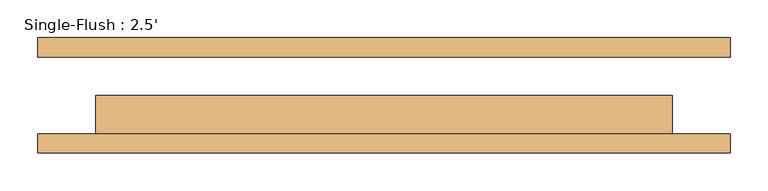
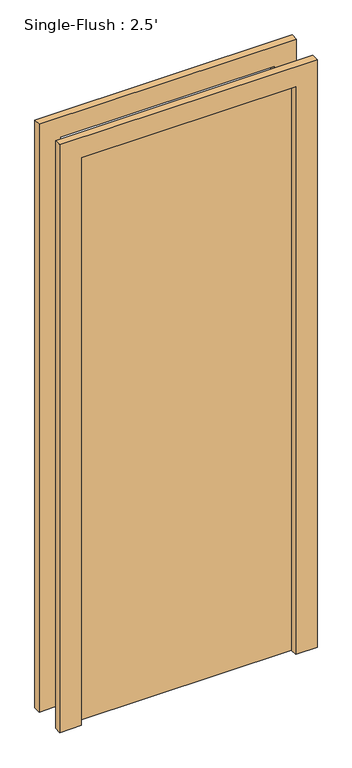
"""IFC4 building model written with IfcOpenShell, lengths in millimetres: door geometry, Single-Flush : 2.5'."""

from ifc_helpers import new_model, si_unit, frame, origin, origin_with_axes, place, context, project, spatial, polyline, outline, extrude, source, transform, mapped, element, save


def single_flush_2_5_aa9e95e7(model_context):
    return source(origin(), model_context, "Body", "SweptSolid", [
        extrude(outline(polyline([(2209.8, -457.2), (0.0, -457.2), (0.0, -381.0), (2133.6, -381.0), (2133.6, 381.0), (0.0, 381.0), (0.0, 457.2), (2209.8, 457.2), (2209.8, -457.2)])), frame((0.0, -76.2, 0.0), z_axis=(0.0, 1.0, 0.0), x_axis=(0.0, 0.0, 1.0)), (0.0, 0.0, 1.0), 25.4),
        extrude(outline(polyline([(2209.8, 457.2), (2209.8, -457.2), (0.0, -457.2), (0.0, -381.0), (2133.6, -381.0), (2133.6, 381.0), (0.0, 381.0), (0.0, 457.2), (2209.8, 457.2)])), frame((0.0, 50.8, 0.0), z_axis=(0.0, 1.0, 0.0), x_axis=(0.0, 0.0, 1.0)), (0.0, 0.0, 1.0), 25.4),
        extrude(outline(polyline([(381.0, 0.0), (381.0, -50.8), (-381.0, -50.8), (-381.0, 0.0), (381.0, 0.0)])), origin_with_axes(), (0.0, 0.0, 1.0), 2133.6),
    ])


if __name__ == "__main__":
    model = new_model("IFC4")
    model_context = context("Model", 3, world=origin())
    ifc_project = project(units=[si_unit("LENGTHUNIT", "METRE", prefix="MILLI")], contexts=[model_context])
    site = spatial("IfcSite", under=ifc_project)
    building = spatial("IfcBuilding", under=site)
    placement = place(None, origin())
    single_flush_2_5_shape = single_flush_2_5_aa9e95e7(model_context)
    element("IfcDoor", 1, ObjectType="Single-Flush : 2.5'", at=placement, inside=building, context=model_context, shape_type="MappedRepresentation", body=[
        mapped(single_flush_2_5_shape, transform((0.0, 0.0, 0.0), x_axis=(1.0, 0.0, 0.0), y_axis=(0.0, 1.0, 0.0), z_axis=(0.0, 0.0, 1.0))),
    ])
    save(model, "model.ifc")

# Revit data of these elements
# Type "Single-Flush : 2.5'"
#   Type Mark = "9"
#   Construction Type Id = "MDOOR"
#   Assembly Code = "C1020"
#   Analytic Construction = "Metal"
#   Thickness = 0' - 2"
#   Heat Transfer Coefficient (U) = 0.651978 BTU/(h·ft²·°F)
#   Height = 7' - 0"
#   Trim Projection Ext = 0' - 1"
#   Trim Projection Int = 0' - 1"
#   Trim Width = 0' - 3"
#   Width = 2' - 6"
#   Define Thermal Properties by = 1
#   Door Material = Door - Panel
#   Frame Material = Door - Frame
#   Visual Light Transmittance = 0
#   Solar Heat Gain Coefficient = 0
#   Function = (empty or 0)
#   Wall Closure = (empty or 0)
# Element 1 (IfcDoor, "Single-Flush : 2.5'")
#   Materials on its faces: "Door - Frame", "Door - Panel"
# Materials
#   "Door - Panel": class "Wood", colour RGB 210 159 95, transparency 0
#   "Door - Frame": colour RGB 118 70 51, transparency 0
